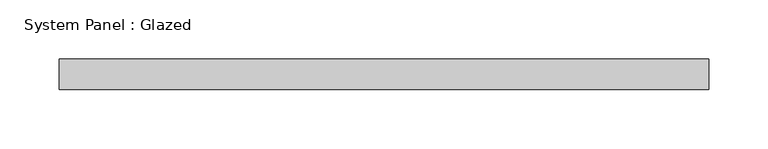
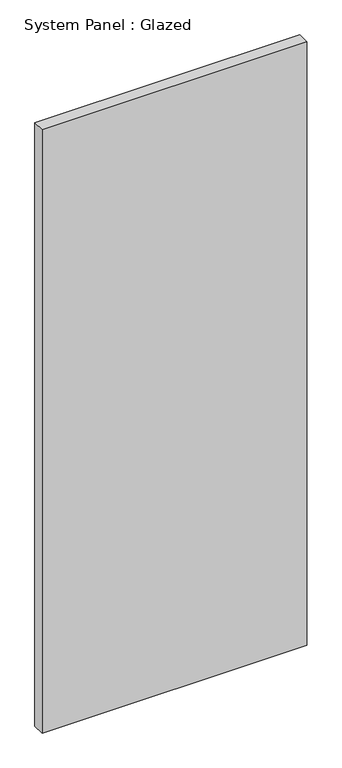
"""IFC4 building model written with IfcOpenShell, lengths in millimetres: plate geometry, System Panel : Glazed."""

from ifc_helpers import new_model, si_unit, origin, origin_with_axes, place, context, project, spatial, polyline, outline, extrude, source, transform, mapped, element, save


def system_panel_glazed_6a6571f5(model_context):
    return source(origin(), model_context, "Body", "SweptSolid", [
        extrude(outline(polyline([(273.05, 19.05), (-273.05, 19.05), (-273.05, 44.45), (273.05, 44.45), (273.05, 19.05)])), origin_with_axes(), (0.0, 0.0, 1.0), 1314.7145247),
    ])


if __name__ == "__main__":
    model = new_model("IFC4")
    model_context = context("Model", 3, world=origin())
    ifc_project = project(units=[si_unit("LENGTHUNIT", "METRE", prefix="MILLI")], contexts=[model_context])
    site = spatial("IfcSite", under=ifc_project)
    building = spatial("IfcBuilding", under=site)
    placement = place(None, origin())
    system_panel_glazed_shape = system_panel_glazed_6a6571f5(model_context)
    element("IfcPlate", 1, ObjectType="System Panel : Glazed", at=placement, inside=building, context=model_context, shape_type="MappedRepresentation", body=[
        mapped(system_panel_glazed_shape, transform((0.0, 0.0, 0.0), x_axis=(1.0, 0.0, 0.0), y_axis=(0.0, 1.0, 0.0), z_axis=(0.0, 0.0, 1.0))),
    ])
    save(model, "model.ifc")

# Revit data of these elements
# Type "System Panel : Glazed"
#   Construction Type Id = "GSP4R"
#   Analytic Construction = "1/8 in Pilkington single glazing"
#   Visual Light Transmittance = 0.9
#   Solar Heat Gain Coefficient = 0.86
#   Heat Transfer Coefficient (U) = 1.18115 BTU/(h·ft²·°F)
#   Define Thermal Properties by = 1
# Element 1 (IfcPlate, "System Panel : Glazed")
#   Materials on its faces: "Glass"
# Materials
#   "Glass": class "Glass", colour RGB 0 128 192, transparency 0.75, Description = "Soda Lime Glass", Cost = 0
